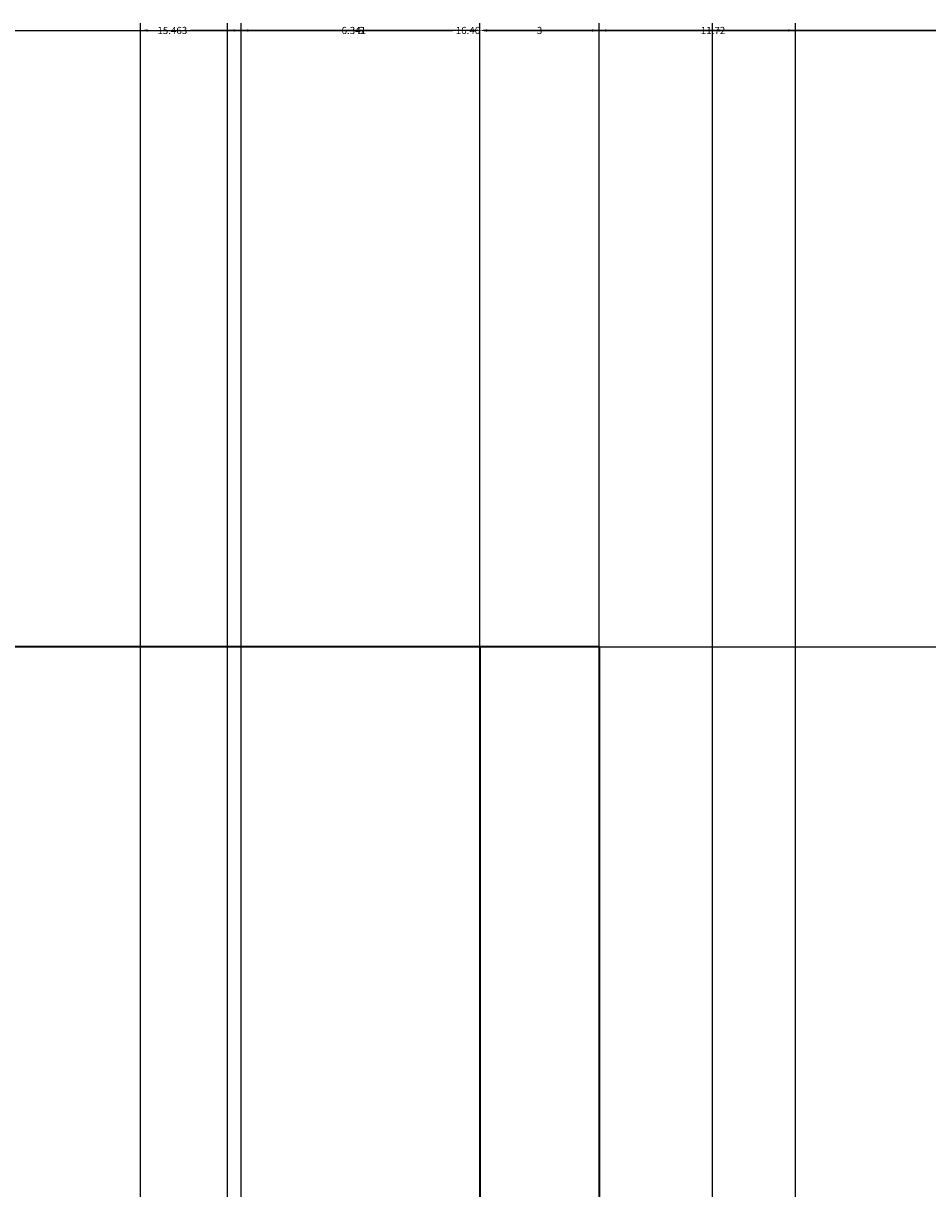
# Model space of a CAD drawing. Units: inches. Extents: x -6 to 289, y -8 to 323.
# Tile 87 of 107: x 104 to 126, y 294 to 323. Entities that reach past the tile are written whole.
import ezdxf

# ---------------------------------------------------------------- set-up
doc = ezdxf.new("R2010")
doc.units = ezdxf.units.IN
doc.header["$MEASUREMENT"] = 0
doc.layers.add('A-ANNO-DIMS', color=2, linetype='Continuous', lineweight=18)
doc.layers.add('A-ELEV', color=7, linetype='Continuous', lineweight=35)
doc.styles.get("Standard").update_dxf_attribs({"font": 'arial.ttf'})
doc.dimstyles.get("Standard").update_dxf_attribs({"dimtxt": 0.18, "dimasz": 0.18, "dimexe": 0.18, "dimexo": 0.0625, "dimgap": 0.09, "dimtad": 0, "dimtih": 1, "dimtoh": 1, "dimdec": 4, "dimzin": 0, "dimdsep": 46, "dimtxsty": 'Standard', "dimcen": 0.09, "dimadec": 0, "dimazin": 0, "dimtfac": 1, "dimtdec": 4, "dimtofl": 0, "dimtmove": 0, "dimatfit": 3, "dimfxl": 1, "dimtolj": 1, "dimtzin": 0, "dimarcsym": 0})

# ---------------------------------------------------------------- blocks, each defined once
blk = doc.blocks.new('*D9')
at = {"layer": 'A-ANNO-DIMS', "color": 0, "lineweight": -2, "transparency": 16777216}
for p, q in [((99.701, 289.105), (99.701, 322.969)), ((115.164, 307.351), (115.164, 322.969)), ((99.881, 322.789), (106.977, 322.789)), ((114.984, 322.789), (107.887, 322.789))]:
    blk.add_line(p, q, dxfattribs=at)
at = {"layer": 'A-ANNO-DIMS', "color": 0, "transparency": 16777216}
for points in [[(99.881, 322.819), (99.881, 322.759), (99.701, 322.789)], [(114.984, 322.819), (114.984, 322.759), (115.164, 322.789)]]:
    blk.add_solid(points, dxfattribs=at)
at = {"layer": 'Defpoints', "color": 0, "transparency": 16777216}
for p in [(115.164, 322.789), (115.164, 307.289), (99.701, 289.043)]:
    blk.add_point(p, dxfattribs=at)
at = {"layer": 'A-ANNO-DIMS', "color": 0, "transparency": 16777216, "insert": (107.432, 322.789), "char_height": 0.18, "attachment_point": 5}
blk.add_mtext('\\A1;15.463', dxfattribs=at)
blk = doc.blocks.new('*D10')
at = {"layer": 'A-ANNO-DIMS', "color": 0, "lineweight": -2, "transparency": 16777216}
for p, q in [((115.164, 307.351), (115.164, 322.969)), ((126.883, 226.717), (126.883, 322.969)), ((115.344, 322.789), (120.639, 322.789)), ((126.703, 322.789), (121.408, 322.789))]:
    blk.add_line(p, q, dxfattribs=at)
at = {"layer": 'A-ANNO-DIMS', "color": 0, "transparency": 16777216}
for points in [[(115.344, 322.819), (115.344, 322.759), (115.164, 322.789)], [(126.703, 322.819), (126.703, 322.759), (126.883, 322.789)]]:
    blk.add_solid(points, dxfattribs=at)
at = {"layer": 'Defpoints', "color": 0, "transparency": 16777216}
for p in [(126.883, 322.789), (115.164, 307.289), (126.883, 226.654)]:
    blk.add_point(p, dxfattribs=at)
at = {"layer": 'A-ANNO-DIMS', "color": 0, "transparency": 16777216, "insert": (121.024, 322.789), "char_height": 0.18, "attachment_point": 5}
blk.add_mtext('\\A1;11.72', dxfattribs=at)
blk = doc.blocks.new('*D27')
at = {"layer": 'A-ANNO-DIMS', "color": 0, "lineweight": -2, "transparency": 16777216}
for p, q in [((19.226, 307.289), (288.653, 307.289)), ((288.473, 307.109), (288.473, 277.471)), ((288.473, 247.469), (288.473, 277.107)), ((247.226, 247.289), (288.653, 247.289))]:
    blk.add_line(p, q, dxfattribs=at)
at = {"layer": 'A-ANNO-DIMS', "color": 0, "transparency": 16777216}
for points in [[(288.443, 307.109), (288.503, 307.109), (288.473, 307.289)], [(288.443, 247.469), (288.503, 247.469), (288.473, 247.289)]]:
    blk.add_solid(points, dxfattribs=at)
at = {"layer": 'Defpoints', "color": 0, "transparency": 16777216}
for p in [(19.164, 307.289), (288.473, 307.289), (247.164, 247.289)]:
    blk.add_point(p, dxfattribs=at)
at = {"layer": 'A-ANNO-DIMS', "color": 0, "transparency": 16777216, "insert": (288.473, 277.289), "char_height": 0.18, "attachment_point": 5}
blk.add_mtext('\\A1;60', dxfattribs=at)
blk = doc.blocks.new('*D58')
at = {"layer": 'A-ANNO-DIMS', "color": 0, "lineweight": -2, "transparency": 16777216}
for p, q in [((106.634, 68.495), (106.634, 322.969)), ((123.094, 68.495), (123.094, 322.969)), ((106.814, 322.789), (114.479, 322.789)), ((122.914, 322.789), (115.249, 322.789))]:
    blk.add_line(p, q, dxfattribs=at)
at = {"layer": 'A-ANNO-DIMS', "color": 0, "transparency": 16777216}
for points in [[(106.814, 322.819), (106.814, 322.759), (106.634, 322.789)], [(122.914, 322.819), (122.914, 322.759), (123.094, 322.789)]]:
    blk.add_solid(points, dxfattribs=at)
at = {"layer": 'Defpoints', "color": 0, "transparency": 16777216}
for p in [(123.094, 322.789), (106.634, 68.432), (123.094, 68.432)]:
    blk.add_point(p, dxfattribs=at)
at = {"layer": 'A-ANNO-DIMS', "color": 0, "transparency": 16777216, "insert": (114.864, 322.789), "char_height": 0.18, "attachment_point": 5}
blk.add_mtext('\\A1;16.46', dxfattribs=at)
blk = doc.blocks.new('*D73')
at = {"layer": 'A-ANNO-DIMS', "color": 0, "lineweight": -2, "transparency": 16777216}
for p, q in [((121.008, 51.148), (121.008, 322.969)), ((135.296, 51.148), (135.296, 322.969)), ((121.188, 322.789), (127.697, 322.789)), ((135.116, 322.789), (128.607, 322.789))]:
    blk.add_line(p, q, dxfattribs=at)
at = {"layer": 'A-ANNO-DIMS', "color": 0, "transparency": 16777216}
for points in [[(121.188, 322.819), (121.188, 322.759), (121.008, 322.789)], [(135.116, 322.819), (135.116, 322.759), (135.296, 322.789)]]:
    blk.add_solid(points, dxfattribs=at)
at = {"layer": 'Defpoints', "color": 0, "transparency": 16777216}
for p in [(135.296, 322.789), (121.008, 51.085), (135.296, 51.085)]:
    blk.add_point(p, dxfattribs=at)
at = {"layer": 'A-ANNO-DIMS', "color": 0, "transparency": 16777216, "insert": (128.152, 322.789), "char_height": 0.18, "attachment_point": 5}
blk.add_mtext('\\A1;14.288', dxfattribs=at)
blk = doc.blocks.new('*D92')
at = {"layer": 'A-ANNO-DIMS', "color": 0, "lineweight": -2, "transparency": 16777216}
for p, q in [((109.164, 127.351), (109.164, 322.969)), ((115.164, 162.411), (115.164, 322.969)), ((109.344, 322.789), (112.014, 322.789)), ((114.984, 322.789), (112.313, 322.789))]:
    blk.add_line(p, q, dxfattribs=at)
at = {"layer": 'A-ANNO-DIMS', "color": 0, "transparency": 16777216}
for points in [[(109.344, 322.819), (109.344, 322.759), (109.164, 322.789)], [(114.984, 322.819), (114.984, 322.759), (115.164, 322.789)]]:
    blk.add_solid(points, dxfattribs=at)
at = {"layer": 'Defpoints', "color": 0, "transparency": 16777216}
for p in [(115.164, 322.789), (115.164, 162.348), (109.164, 127.289)]:
    blk.add_point(p, dxfattribs=at)
at = {"layer": 'A-ANNO-DIMS', "color": 0, "transparency": 16777216, "insert": (112.164, 322.789), "char_height": 0.18, "attachment_point": 5}
blk.add_mtext('\\A1;6', dxfattribs=at)
blk = doc.blocks.new('*D93')
at = {"layer": 'A-ANNO-DIMS', "color": 0, "lineweight": -2, "transparency": 16777216}
for p, q in [((115.164, 162.411), (115.164, 322.969)), ((118.164, 159.411), (118.164, 322.969)), ((115.344, 322.789), (116.515, 322.789)), ((117.984, 322.789), (116.813, 322.789))]:
    blk.add_line(p, q, dxfattribs=at)
at = {"layer": 'A-ANNO-DIMS', "color": 0, "transparency": 16777216}
for points in [[(115.344, 322.819), (115.344, 322.759), (115.164, 322.789)], [(117.984, 322.819), (117.984, 322.759), (118.164, 322.789)]]:
    blk.add_solid(points, dxfattribs=at)
at = {"layer": 'Defpoints', "color": 0, "transparency": 16777216}
for p in [(118.164, 322.789), (115.164, 162.348), (118.164, 159.348)]:
    blk.add_point(p, dxfattribs=at)
at = {"layer": 'A-ANNO-DIMS', "color": 0, "transparency": 16777216, "insert": (116.664, 322.789), "char_height": 0.18, "attachment_point": 5}
blk.add_mtext('\\A1;3', dxfattribs=at)
blk = doc.blocks.new('*D94')
at = {"layer": 'A-ANNO-DIMS', "color": 0, "lineweight": -2, "transparency": 16777216}
for p, q in [((118.164, 159.411), (118.164, 322.969)), ((161.552, 159.411), (161.552, 322.969)), ((118.344, 322.789), (139.46, 322.789)), ((161.372, 322.789), (140.256, 322.789))]:
    blk.add_line(p, q, dxfattribs=at)
at = {"layer": 'A-ANNO-DIMS', "color": 0, "transparency": 16777216}
for points in [[(118.344, 322.819), (118.344, 322.759), (118.164, 322.789)], [(161.372, 322.819), (161.372, 322.759), (161.552, 322.789)]]:
    blk.add_solid(points, dxfattribs=at)
at = {"layer": 'Defpoints', "color": 0, "transparency": 16777216}
for p in [(161.552, 322.789), (118.164, 159.348), (161.552, 159.348)]:
    blk.add_point(p, dxfattribs=at)
at = {"layer": 'A-ANNO-DIMS', "color": 0, "transparency": 16777216, "insert": (139.858, 322.789), "char_height": 0.18, "attachment_point": 5}
blk.add_mtext('\\A1;43.39', dxfattribs=at)
blk = doc.blocks.new('*D105')
at = {"layer": 'A-ANNO-DIMS', "color": 0, "lineweight": -2, "transparency": 16777216}
for p, q in [((108.823, 259.351), (108.823, 322.969)), ((115.164, 277.105), (115.164, 322.969)), ((109.003, 322.789), (111.616, 322.789)), ((114.984, 322.789), (112.37, 322.789))]:
    blk.add_line(p, q, dxfattribs=at)
at = {"layer": 'A-ANNO-DIMS', "color": 0, "transparency": 16777216}
for points in [[(109.003, 322.819), (109.003, 322.759), (108.823, 322.789)], [(114.984, 322.819), (114.984, 322.759), (115.164, 322.789)]]:
    blk.add_solid(points, dxfattribs=at)
at = {"layer": 'Defpoints', "color": 0, "transparency": 16777216}
for p in [(115.164, 322.789), (115.164, 277.043), (108.823, 259.289)]:
    blk.add_point(p, dxfattribs=at)
at = {"layer": 'A-ANNO-DIMS', "color": 0, "transparency": 16777216, "insert": (111.993, 322.789), "char_height": 0.18, "attachment_point": 5}
blk.add_mtext('\\A1;6.341', dxfattribs=at)
blk = doc.blocks.new('*D106')
at = {"layer": 'A-ANNO-DIMS', "color": 0, "lineweight": -2, "transparency": 16777216}
for p, q in [((115.164, 277.105), (115.164, 322.969)), ((118.164, 293.728), (118.164, 322.969)), ((115.344, 322.789), (116.515, 322.789)), ((117.984, 322.789), (116.813, 322.789))]:
    blk.add_line(p, q, dxfattribs=at)
at = {"layer": 'A-ANNO-DIMS', "color": 0, "transparency": 16777216}
for points in [[(115.344, 322.819), (115.344, 322.759), (115.164, 322.789)], [(117.984, 322.819), (117.984, 322.759), (118.164, 322.789)]]:
    blk.add_solid(points, dxfattribs=at)
at = {"layer": 'Defpoints', "color": 0, "transparency": 16777216}
for p in [(118.164, 322.789), (118.164, 293.666), (115.164, 277.043)]:
    blk.add_point(p, dxfattribs=at)
at = {"layer": 'A-ANNO-DIMS', "color": 0, "transparency": 16777216, "insert": (116.664, 322.789), "char_height": 0.18, "attachment_point": 5}
blk.add_mtext('\\A1;3', dxfattribs=at)
blk = doc.blocks.new('*D107')
at = {"layer": 'A-ANNO-DIMS', "color": 0, "lineweight": -2, "transparency": 16777216}
for p, q in [((118.164, 293.728), (118.164, 322.969)), ((186.984, 291.541), (186.984, 322.969)), ((118.344, 322.789), (152.18, 322.789)), ((186.804, 322.789), (152.967, 322.789))]:
    blk.add_line(p, q, dxfattribs=at)
at = {"layer": 'A-ANNO-DIMS', "color": 0, "transparency": 16777216}
for points in [[(118.344, 322.819), (118.344, 322.759), (118.164, 322.789)], [(186.804, 322.819), (186.804, 322.759), (186.984, 322.789)]]:
    blk.add_solid(points, dxfattribs=at)
at = {"layer": 'Defpoints', "color": 0, "transparency": 16777216}
for p in [(186.984, 322.789), (118.164, 293.666), (186.984, 291.478)]:
    blk.add_point(p, dxfattribs=at)
at = {"layer": 'A-ANNO-DIMS', "color": 0, "transparency": 16777216, "insert": (152.574, 322.789), "char_height": 0.18, "attachment_point": 5}
blk.add_mtext('\\A1;68.82', dxfattribs=at)
blk = doc.blocks.new('*D118')
at = {"layer": 'A-ANNO-DIMS', "color": 0, "lineweight": -2, "transparency": 16777216}
for p, q in [((118.226, 307.289), (288.653, 307.289)), ((288.473, 307.109), (288.473, 300.659)), ((288.473, 293.846), (288.473, 300.295)), ((257.703, 293.666), (288.653, 293.666))]:
    blk.add_line(p, q, dxfattribs=at)
at = {"layer": 'A-ANNO-DIMS', "color": 0, "transparency": 16777216}
for points in [[(288.443, 307.109), (288.503, 307.109), (288.473, 307.289)], [(288.443, 293.846), (288.503, 293.846), (288.473, 293.666)]]:
    blk.add_solid(points, dxfattribs=at)
at = {"layer": 'Defpoints', "color": 0, "transparency": 16777216}
for p in [(118.164, 307.289), (288.473, 307.289), (257.641, 293.666)]:
    blk.add_point(p, dxfattribs=at)
at = {"layer": 'A-ANNO-DIMS', "color": 0, "transparency": 16777216, "insert": (288.473, 300.477), "char_height": 0.18, "attachment_point": 5}
blk.add_mtext('\\A1;13.623', dxfattribs=at)

msp = doc.modelspace()

# ---------------------------------------------------------------- linework, layer by layer
at = {"layer": 'A-ELEV'}
msp.add_line((118.1638, 307.2888), (19.1638, 307.2888), dxfattribs=at)
for points in [[(115.1638, 307.2888), (115.1638, 277.0427), (259.1638, 277.0427), (259.1638, 259.2888)], [(118.1638, 307.2888), (118.1638, 280.0427), (262.1638, 280.0427), (262.1638, 259.2888)]]:
    msp.add_lwpolyline(points, dxfattribs=at)

# ---------------------------------------------------------------- dimensions: what is measured, and where the dimension line sits
at = {"layer": 'A-ANNO-DIMS'}
for base, p1, p2, override, picture, middle in [((115.1638, 322.7888), (99.7007, 289.0427), (115.1638, 307.2888), {"dimdec": 3, "dimlfac": 1, "dimrnd": 0, "dimzin": 0, "dimdsep": 46, "dimlunit": 2}, '*D9', (107.4322, 322.7888)), ((123.094, 322.7888), (106.634, 68.4322), (123.094, 68.4322), {"dimdec": 2, "dimlfac": 1, "dimrnd": 0, "dimzin": 0, "dimdsep": 46, "dimlunit": 2}, '*D58', (114.864, 322.7888)), ((115.1638, 322.7888), (108.8227, 259.2888), (115.1638, 277.0427), {"dimdec": 3, "dimlfac": 1, "dimrnd": 0, "dimzin": 0, "dimdsep": 46, "dimlunit": 2}, '*D105', (111.9933, 322.7888)), ((115.1638, 322.7888), (109.1638, 127.2888), (115.1638, 162.3484), {"dimdec": 0, "dimlfac": 1, "dimrnd": 0, "dimzin": 0, "dimdsep": 46, "dimlunit": 2}, '*D92', (112.1638, 322.7888)), ((126.8835, 322.7888), (115.1638, 307.2888), (126.8835, 226.654), {"dimdec": 2, "dimlfac": 1, "dimrnd": 0, "dimzin": 0, "dimdsep": 46, "dimlunit": 2}, '*D10', (121.0236, 322.7888)), ((118.1638, 322.7888), (115.1638, 162.3484), (118.1638, 159.3484), {"dimdec": 0, "dimlfac": 1, "dimrnd": 0, "dimzin": 0, "dimdsep": 46, "dimlunit": 2}, '*D93', (116.6638, 322.7888)), ((118.1638, 322.7888), (115.1638, 277.0427), (118.1638, 293.6657), {"dimdec": 0, "dimlfac": 1, "dimrnd": 0, "dimzin": 0, "dimdsep": 46, "dimlunit": 2}, '*D106', (116.6638, 322.7888)), ((161.5522, 322.7888), (118.1638, 159.3484), (161.5522, 159.3484), {"dimdec": 2, "dimlfac": 1, "dimrnd": 0, "dimzin": 0, "dimdsep": 46, "dimlunit": 2}, '*D94', (139.858, 322.7888)), ((186.9837, 322.7888), (118.1638, 293.6657), (186.9837, 291.4781), {"dimdec": 2, "dimlfac": 1, "dimrnd": 0, "dimzin": 0, "dimdsep": 46, "dimlunit": 2}, '*D107', (152.5737, 322.7888)), ((135.296, 322.7888), (121.008, 51.0851), (135.296, 51.0851), {"dimdec": 3, "dimlfac": 1, "dimrnd": 0, "dimzin": 0, "dimdsep": 46, "dimlunit": 2}, '*D73', (128.152, 322.7888))]:
    dim = msp.add_linear_dim(base=base, p1=p1, p2=p2, dimstyle='Standard', override=override, dxfattribs=at)
    dim.commit()
    dim.dimension.update_dxf_attribs({"geometry": picture, "text_midpoint": middle})
for p1, p2, override, picture, middle in [((247.1638, 247.2888), (19.1638, 307.2888), {"dimdec": 0, "dimlfac": 1, "dimrnd": 0, "dimzin": 0, "dimdsep": 46, "dimlunit": 2}, '*D27', (288.4733, 277.2888)), ((257.6407, 293.6657), (118.1638, 307.2888), {"dimdec": 3, "dimlfac": 1, "dimrnd": 0, "dimzin": 0, "dimdsep": 46, "dimlunit": 2}, '*D118', (288.4733, 300.4773))]:
    dim = msp.add_linear_dim(base=(288.4733, 307.2888), p1=p1, p2=p2, angle=90, dimstyle='Standard', override=override, dxfattribs=at)
    dim.commit()
    dim.dimension.update_dxf_attribs({"geometry": picture, "text_midpoint": middle})

doc.saveas('drawing.dxf')
